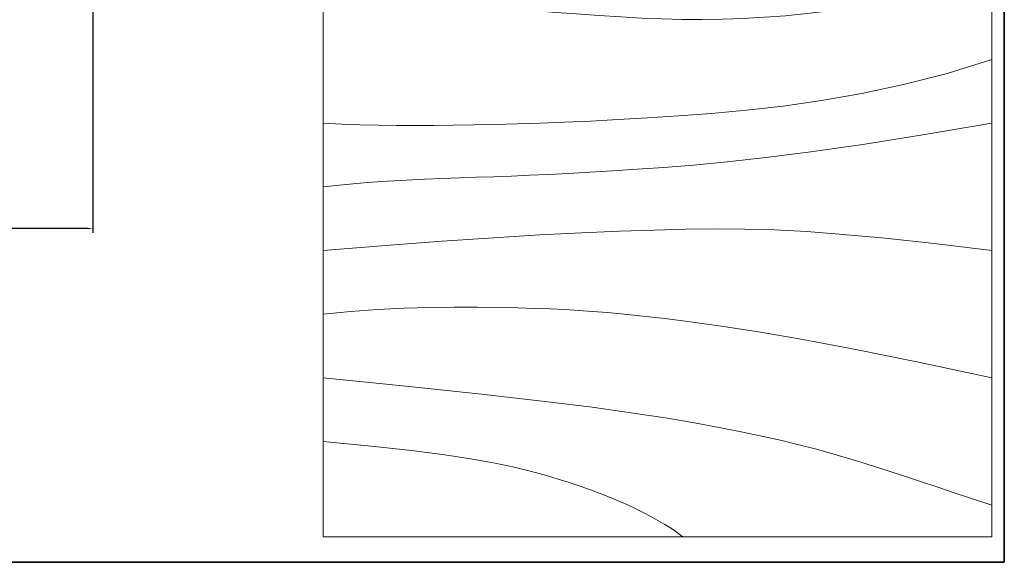
# Model space of a CAD drawing. Units: inches. Extents: x -128 to 854, y -395 to 398.
# Tile 33 of 61: x 265 to 305, y 73 to 95. Entities that reach past the tile are written whole.
import ezdxf

# ---------------------------------------------------------------- set-up
doc = ezdxf.new("R2010")
doc.units = ezdxf.units.IN
doc.header["$MEASUREMENT"] = 0
for name, color, linetype, lineweight in [('A-ANNO-DIMS', 2, 'Continuous', 18), ('A-FURN', 8, 'Continuous', 18), ('A-WALL', 4, 'Continuous', 35)]:
    doc.layers.add(name, color=color, linetype=linetype, lineweight=lineweight)
doc.styles.get("Standard").update_dxf_attribs({"font": 'arial.ttf'})
doc.dimstyles.get("Standard").update_dxf_attribs({"dimtxt": 0.18, "dimasz": 0.18, "dimexe": 0.18, "dimexo": 0.0625, "dimgap": 0.09, "dimtad": 0, "dimtih": 1, "dimtoh": 1, "dimdec": 1, "dimzin": 0, "dimdsep": 46, "dimlunit": 4, "dimtxsty": 'Standard', "dimcen": 0.09, "dimclrd": 1, "dimclre": 2, "dimclrt": 6, "dimadec": 0, "dimazin": 0, "dimtfac": 1, "dimtdec": 1, "dimtofl": 0, "dimtmove": 0, "dimatfit": 3, "dimfxl": 1, "dimtfill": 2, "dimtfillclr": 3, "dimtolj": 1, "dimtzin": 0, "dimarcsym": 0})

# ---------------------------------------------------------------- blocks, each defined once
blk = doc.blocks.new('Table - Square Woodgrain 42 x 42 in.')
blk.add_line((0, -42), (42, -42))
for points in [[(0, -4), (1.704, -4.2172), (3.2358, -4.4188), (4.615, -4.604), (5.8615, -4.7721), (6.9951, -4.9224), (8.0357, -5.0541), (9.0031, -5.1667), (9.9171, -5.2594), (10.7951, -5.3316), (11.6445, -5.3836), (12.4702, -5.4157), (13.277, -5.4283), (14.0698, -5.4217), (14.8535, -5.3964), (15.6331, -5.3526), (16.4133, -5.2908), (17.1986, -5.2103), (17.9913, -5.1062), (18.793, -4.9727), (19.6056, -4.8038), (20.4307, -4.5937), (21.2701, -4.3365), (22.1256, -4.0262), (22.9989, -3.6571), (23.888, -3.2272), (24.7756, -2.7516), (25.6408, -2.2491), (26.4624, -1.7387), (27.2195, -1.2395), (27.891, -0.7703), (28.456, -0.3501), (28.8934, 0.002)], [(0, -42), (0, 0), (42, 0), (42, -42)], [(0, -8), (1.8203, -8.1001), (3.6741, -8.2149), (5.5411, -8.3408), (7.4011, -8.4741), (9.2339, -8.6112), (11.0193, -8.7484), (12.7371, -8.8821), (14.3671, -9.0086), (15.8954, -9.1246), (17.3337, -9.2278), (18.6997, -9.3159), (20.0116, -9.387), (21.2871, -9.4389), (22.5442, -9.4696), (23.8008, -9.477), (25.0749, -9.459), (26.3791, -9.4137), (27.7049, -9.3403), (29.0383, -9.2382), (30.3655, -9.1068), (31.6728, -8.9455), (32.9461, -8.7535), (34.1717, -8.5304), (35.3358, -8.2756), (36.4268, -7.9863), (37.443, -7.6521), (38.3849, -7.2603), (39.253, -6.7986), (40.048, -6.2542), (40.7705, -5.6147), (41.421, -4.8674), (42, -4)], [(42, -12), (39.1784, -12.8621), (36.4519, -13.5654), (33.8246, -14.1294), (31.3004, -14.5731), (28.8832, -14.9161), (26.577, -15.1775), (24.3858, -15.3768), (22.3136, -15.5332), (20.3622, -15.6632), (18.5254, -15.7718), (16.7947, -15.8612), (15.1618, -15.9338), (13.6183, -15.9916), (12.1558, -16.0369), (10.7659, -16.0718), (9.4403, -16.0987), (8.1703, -16.1191), (6.9461, -16.1325), (5.7577, -16.1377), (4.595, -16.1335), (3.4479, -16.1188), (2.3064, -16.0924), (1.1604, -16.0532), (0, -16)], [(42, -16), (37.6529, -16.7365), (33.8802, -17.329), (30.6179, -17.7961), (27.8015, -18.1561), (25.3668, -18.4275), (23.2497, -18.6288), (21.3859, -18.7785), (19.7111, -18.8949), (18.1693, -18.9939), (16.7375, -19.0795), (15.401, -19.1534), (14.1449, -19.217), (12.9544, -19.2717), (11.8148, -19.3191), (10.7113, -19.3606), (9.6291, -19.3976), (8.5534, -19.4323), (7.47, -19.4689), (6.3643, -19.5122), (5.222, -19.5672), (4.0288, -19.6386), (2.7703, -19.7313), (1.4321, -19.8501), (0, -20)], [(0, -24), (3.9243, -23.6805), (7.4766, -23.4138), (10.6891, -23.1954), (13.5943, -23.0205), (16.2247, -22.8847), (18.6125, -22.7832), (20.7903, -22.7116), (22.7903, -22.6651), (24.6563, -22.642), (26.4764, -22.6507), (28.35, -22.7024), (30.3766, -22.8084), (32.6555, -22.98), (35.2861, -23.2283), (38.3678, -23.5645), (42, -24)], [(42, -32), (37.392, -31.017), (33.4585, -30.2231), (30.1291, -29.5949), (27.3334, -29.109), (25.0009, -28.742), (23.0612, -28.4707), (21.4439, -28.2716), (20.0786, -28.1215), (18.8998, -28.0002), (17.8609, -27.9014), (16.9206, -27.8219), (16.0371, -27.7588), (15.1691, -27.709), (14.2748, -27.6693), (13.3128, -27.6368), (12.2415, -27.6083), (11.0295, -27.5824), (9.6867, -27.5643), (8.233, -27.5608), (6.6884, -27.5787), (5.0728, -27.6248), (3.4062, -27.7058), (1.7086, -27.8286), (0, -28)], [(0, -32), (5.4026, -32.5358), (9.9494, -33.019), (13.7424, -33.4553), (16.8834, -33.8505), (19.4743, -34.2106), (21.6171, -34.5413), (23.4136, -34.8486), (24.9657, -35.1382), (26.3614, -35.4156), (27.6332, -35.6841), (28.7995, -35.9467), (29.8788, -36.2064), (30.8897, -36.4661), (31.8507, -36.7288), (32.7802, -36.9973), (33.6968, -37.2747), (34.6175, -37.5635), (35.5531, -37.8651), (36.5128, -38.1805), (37.506, -38.5108), (38.5421, -38.8568), (39.6302, -39.2197), (40.7797, -39.6004), (42, -40)], [(0, -36), (3.0098, -36.2857), (5.5354, -36.5643), (7.6368, -36.8359), (9.374, -37.1009), (10.807, -37.3597), (11.9957, -37.6126), (13.0002, -37.8599), (13.8804, -38.102), (14.6874, -38.3393), (15.4365, -38.5729), (16.1338, -38.8041), (16.7858, -39.0341), (17.3987, -39.264), (17.9787, -39.4952), (18.5322, -39.7288), (19.0655, -39.9662), (19.5832, -40.2081), (20.0842, -40.4544), (20.5657, -40.7046), (21.0249, -40.9581), (21.459, -41.2144), (21.8653, -41.4731), (22.2409, -41.7335), (22.5831, -41.9951)]]:
    blk.add_lwpolyline(points)
blk = doc.blocks.new('*D55')
at = {"layer": 'A-ANNO-DIMS', "color": 0, "lineweight": -2, "transparency": 16777216}
for p, q in [((304.81, 186.741), (221.092, 186.741)), ((221.272, 181.741), (221.272, 131.873)), ((221.272, 77.741), (221.272, 127.608)), ((304.81, 72.741), (221.092, 72.741))]:
    blk.add_line(p, q, dxfattribs=at)
at = {"layer": 'A-ANNO-DIMS', "color": 0, "transparency": 16777216}
for points in [[(220.439, 181.741), (222.105, 181.741), (221.272, 186.741)], [(220.439, 77.741), (222.105, 77.741), (221.272, 72.741)]]:
    blk.add_solid(points, dxfattribs=at)
at = {"layer": 'Defpoints', "color": 0, "transparency": 16777216}
for p in [(221.272, 186.741), (304.873, 186.741), (304.873, 72.741)]:
    blk.add_point(p, dxfattribs=at)
at = {"layer": 'A-ANNO-DIMS', "color": 0, "transparency": 16777216, "insert": (221.272, 129.741), "char_height": 4, "attachment_point": 5, "bg_fill": 1, "box_fill_scale": 1.25, "bg_fill_color": 3, "bg_fill_transparency": 0}
blk.add_mtext('\\A1;9\'-6"', dxfattribs=at)
blk = doc.blocks.new('*D92')
at = {"layer": 'A-ANNO-DIMS', "color": 2, "lineweight": -2, "transparency": 16777216}
for p, q in [((229.83, 95.667), (229.83, 86.089)), ((267.948, 95.667), (267.948, 86.089))]:
    blk.add_line(p, q, dxfattribs=at)
at = {"layer": 'A-ANNO-DIMS', "color": 1, "lineweight": -2, "transparency": 16777216}
for p, q in [((230.01, 86.269), (248.56, 86.269)), ((267.768, 86.269), (249.218, 86.269))]:
    blk.add_line(p, q, dxfattribs=at)
at = {"layer": 'A-ANNO-DIMS', "color": 1, "transparency": 16777216}
for points in [[(230.01, 86.299), (230.01, 86.239), (229.83, 86.269)], [(267.768, 86.299), (267.768, 86.239), (267.948, 86.269)]]:
    blk.add_solid(points, dxfattribs=at)
at = {"layer": 'Defpoints', "color": 0, "transparency": 16777216}
for p in [(229.83, 95.73), (267.948, 95.73), (267.948, 86.269)]:
    blk.add_point(p, dxfattribs=at)
at = {"layer": 'A-ANNO-DIMS', "color": 6, "transparency": 16777216, "insert": (248.889, 86.269), "char_height": 0.18, "attachment_point": 5, "bg_fill": 1, "box_fill_scale": 1.25, "bg_fill_color": 3, "bg_fill_transparency": 0}
blk.add_mtext('\\A1;3\'-2"', dxfattribs=at)

msp = doc.modelspace()

# ---------------------------------------------------------------- linework, layer by layer
at = {"layer": 'A-WALL'}
for p, q in [((304.873, 186.741), (304.873, 72.741)), ((304.873, 72.741), (196.42, 72.741))]:
    msp.add_line(p, q, dxfattribs=at)

# ---------------------------------------------------------------- block references
at = {"layer": 'A-FURN', "xscale": 0.6449685946951323, "yscale": 0.6449685946951323, "zscale": 0.6449685946951323}
msp.add_blockref('Table - Square Woodgrain 42 x 42 in.', (277.284, 100.856), dxfattribs=at)

# ---------------------------------------------------------------- dimensions: what is measured, and where the dimension line sits
at = {"layer": 'A-ANNO-DIMS'}
dim = msp.add_linear_dim(base=(221.272, 186.741), p1=(304.873, 72.741), p2=(304.873, 186.741), angle=90, dimstyle='Standard', override={"dimtxt": 4, "dimasz": 5, "dimclrd": 0, "dimclre": 0, "dimclrt": 0}, dxfattribs=at)
dim.commit()
dim.dimension.update_dxf_attribs({"geometry": '*D55', "text_midpoint": (221.272, 129.741)})
dim = msp.add_linear_dim(base=(267.948, 86.269), p1=(229.83, 95.73), p2=(267.948, 95.73), dimstyle='Standard', override={"dimdec": 1, "dimlfac": 1, "dimrnd": 0, "dimzin": 1, "dimdsep": 46, "dimlunit": 4, "dimfrac": 2}, dxfattribs=at)
dim.commit()
dim.dimension.update_dxf_attribs({"geometry": '*D92', "text_midpoint": (248.889, 86.269)})

doc.saveas('drawing.dxf')
